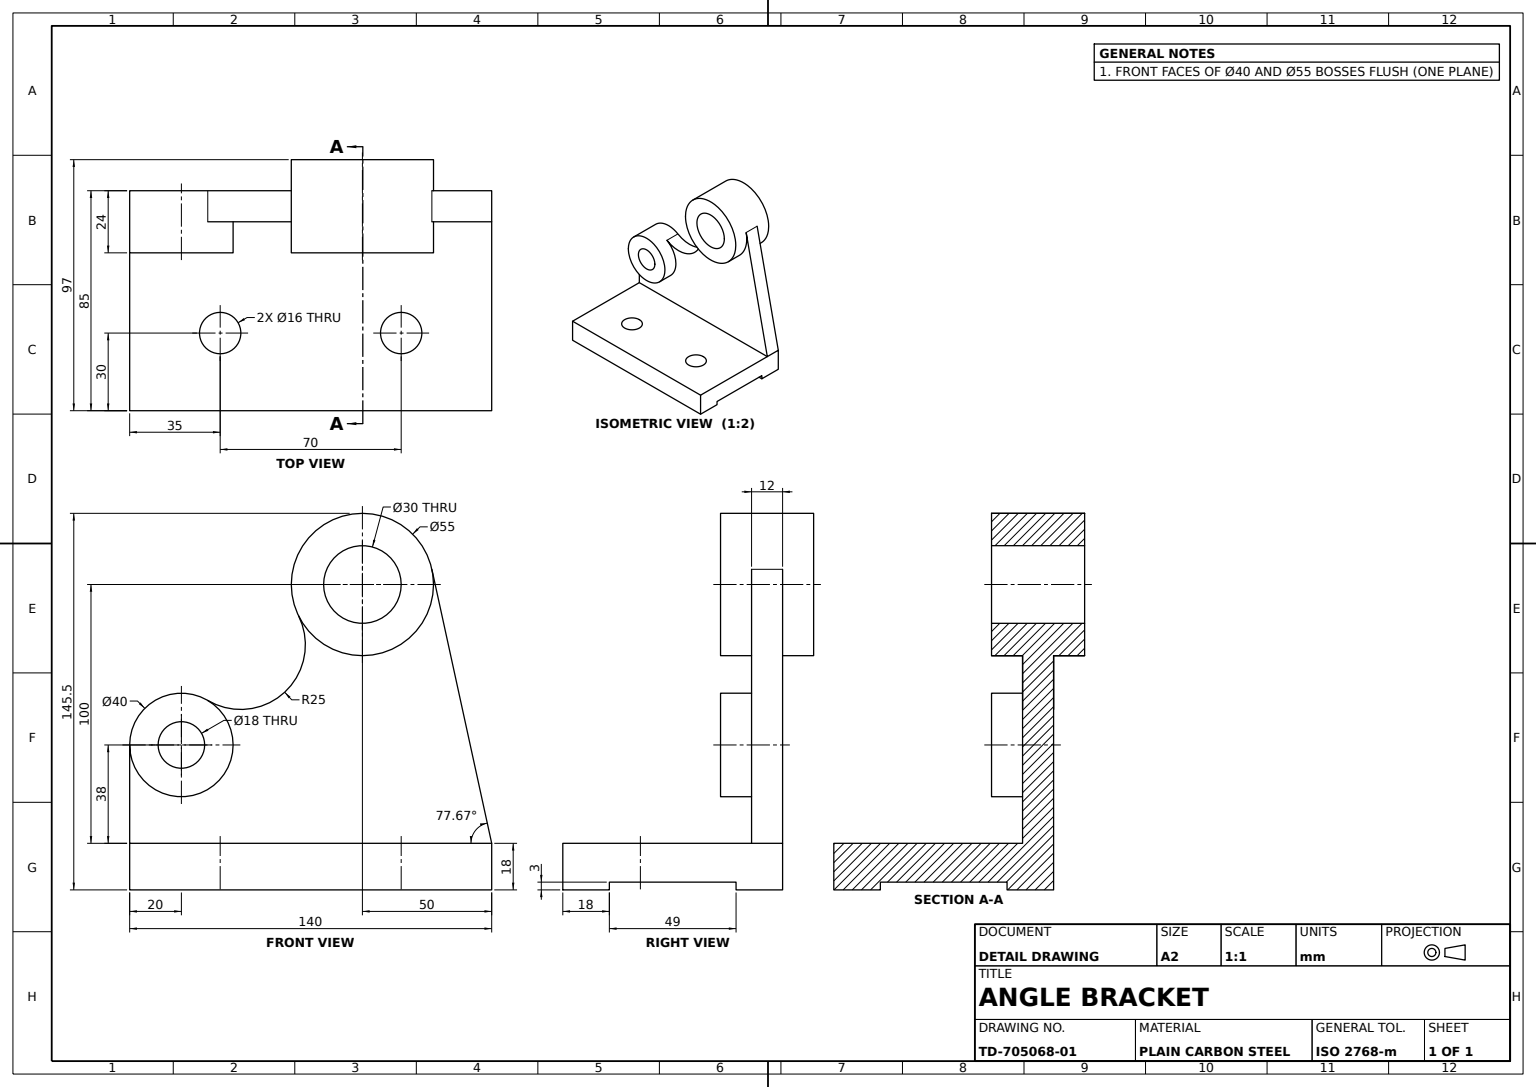
SolidWorks part; units mm, degrees
material "Plain Carbon Steel"
ref_plane "Front Plane" through (0, 0, 0) normal (0, 0, 1) x (1, 0, 0)
ref_plane "Top Plane" through (0, 0, 0) normal (0, 1, 0) x (1, 0, 0)
ref_plane "Right Plane" through (0, 0, 0) normal (1, 0, 0) x (0, 0, -1)
sketch "Base Plate Sketch" plane through (0, 0, 0) normal (0, 1, 0) x (1, 0, 0)
  line L1 (-70, -42.5) -> (70, -42.5)
  line L2 (-70, -42.5) -> (-70, 42.5)
  line L3 (-70, 42.5) -> (70, 42.5)
  line L4 (70, -42.5) -> (70, 42.5)
  line L5 (-70, -42.5) -> (70, 42.5) construction
  line L6 (-70, 42.5) -> (70, -42.5) construction
  point P0 (0, 0)
  dimension "D1" = 140
  dimension "D2" = 85
extrude "Base Plate" add sketch "Base Plate Sketch" along normal blind 18
sketch "Underside Groove Sketch" plane through (70, 0, 0) normal (1, 0, 0) x (0, 0, -1)
  line L0 (-42.5, 0) -> (42.5, 0) construction
  line L1 (-24.5, 0) -> (24.5, 0)
  line L2 (-24.5, 0) -> (-24.5, 3)
  line L3 (-24.5, 3) -> (24.5, 3)
  line L4 (24.5, 0) -> (24.5, 3)
  line L5 (42.5, 18) -> (42.5, 0) construction
  line L6 (-42.5, 18) -> (-42.5, 0) construction
  dimension "D1" = 3
  dimension "D2" = 18
  dimension "D3" = 18
extrude "Underside Groove" cut sketch "Underside Groove Sketch" against normal through all
sketch "Base Holes Sketch" plane through (0, 18, 0) normal (0, 1, 0) x (1, 0, 0)
  line L0 (0, 49.6581) -> (0, -52.4169) construction
  line L1 (-70, 42.5) -> (-70, -42.5) construction
  line L2 (-70, -42.5) -> (70, -42.5) construction
  circle A0 centre (-35, -12.5) radius 8
  circle A1 centre (35, -12.5) radius 8
  dimension "D4" = 16
  dimension "D1" = 35
  dimension "D2" = 70
  dimension "D3" = 30
extrude "Base Holes" cut sketch "Base Holes Sketch" against normal through all
sketch "Upright Lug Plate Sketch" plane through (0, 0, -42.5) normal (0, 0, -1) x (-1, 0, 0)
  line L0 (-70, 18) -> (-20, 18) construction
  line L1 (-70, 18) -> (70, 18) construction
  line L2 (-20, 18) -> (-20, 118) construction
  line L3 (-20, 118) -> (20, 118) construction
  line L4 (20, 118) -> (20, 18) construction
  line L5 (20, 18) -> (70, 18) construction
  circle A0 centre (-20, 118) radius 27.5
  circle A1 centre (-20, 118) radius 15
  dimension "D5" = 55
  dimension "D6" = 55
  dimension "D7" = 30
  dimension "D1" = 50
  dimension "D2" = 100
  dimension "D3" = 100
  dimension "D4" = 50
extrude "Upright Lug Plate" add sketch "Upright Lug Plate Sketch" along normal blind 12 and the other way blind 24 separate body
sketch "Side Gusset Sketch" plane through (0, 0, -42.5) normal (0, 0, -1) x (-1, 0, 0)
  line L0 (70, 18) -> (50, 18) construction
  line L1 (-70, 18) -> (70, 18) construction
  line L2 (50, 18) -> (50, 56) construction
  circle A0 centre (50, 56) radius 20
  circle A1 centre (50, 56) radius 9
  dimension "D3" = 18
  dimension "D4" = 40
  dimension "D1" = 20
  dimension "D2" = 38
extrude "Side Gusset" add sketch "Side Gusset Sketch" against normal blind 24 separate body
sketch "Hinge Boss Extension Sketch" plane through (0, 0, -42.5) normal (0, 0, -1) x (-1, 0, 0)
  line L0 (70, 18) -> (70, 56)
  line L1 (-70, 18) -> (-46.8661, 123.8705)
  line L4 (-70, 0) -> (70, 0)
  line L5 (70, 0) -> (70, 18)
  line L6 (70, 18) -> (-70, 18)
  line L7 (-70, 18) -> (-70, 0)
  line L10 (70, 18) -> (-70, 18)
  circle A1 centre (50, 56) radius 20
  arc A2 (39.8002, 73.2036) -> (70, 56) centre (50, 56) ccw
  circle A3 centre (-20, 118) radius 27.5
  arc A4 (-46.8661, 123.8705) -> (4.6454, 105.7995) centre (-20, 118) ccw
  arc A6 (4.6454, 105.7995) -> (39.8002, 73.2036) centre (27.0503, 94.7081) ccw
  dimension "D4" = 25
  dimension "D1" = 0
  dimension "D2" = 0
  dimension "D3" = 0
extrude "Hinge Boss Extension" add sketch "Hinge Boss Extension Sketch" against normal blind 12
